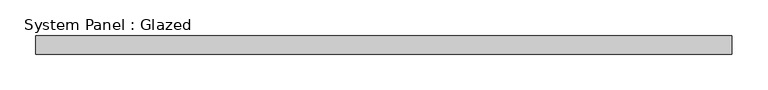
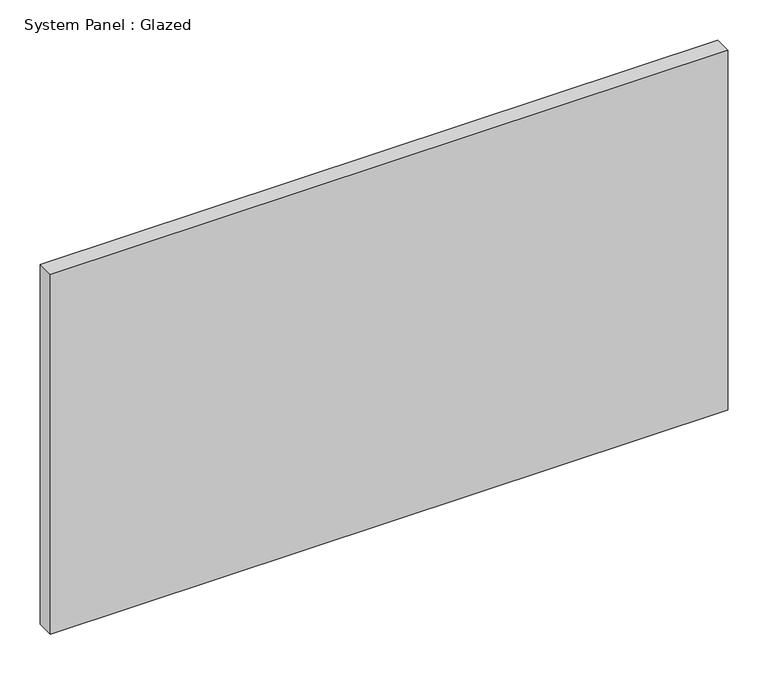
"""IFC4 building model written with IfcOpenShell, lengths in millimetres: plate geometry, System Panel : Glazed."""

from ifc_helpers import new_model, si_unit, origin, origin_with_axes, place, context, project, spatial, polyline, outline, extrude, source, transform, mapped, element, save


def system_panel_glazed_55a8196a(model_context):
    return source(origin(), model_context, "Body", "SweptSolid", [
        extrude(outline(polyline([(485.775, 19.05), (-485.775, 19.05), (-485.775, 44.45), (485.775, 44.45), (485.775, 19.05)])), origin_with_axes(), (0.0, 0.0, 1.0), 546.1),
    ])


if __name__ == "__main__":
    model = new_model("IFC4")
    model_context = context("Model", 3, world=origin())
    ifc_project = project(units=[si_unit("LENGTHUNIT", "METRE", prefix="MILLI")], contexts=[model_context])
    site = spatial("IfcSite", under=ifc_project)
    building = spatial("IfcBuilding", under=site)
    placement = place(None, origin())
    system_panel_glazed_shape = system_panel_glazed_55a8196a(model_context)
    element("IfcPlate", 1, ObjectType="System Panel : Glazed", at=placement, inside=building, context=model_context, shape_type="MappedRepresentation", body=[
        mapped(system_panel_glazed_shape, transform((0.0, 0.0, 0.0), x_axis=(1.0, 0.0, 0.0), y_axis=(0.0, 1.0, 0.0), z_axis=(0.0, 0.0, 1.0))),
    ])
    save(model, "model.ifc")

# Revit data of these elements
# Type "System Panel : Glazed"
#   Construction Type Id = "GSP4R"
#   Analytic Construction = "1/8 in Pilkington single glazing"
#   Visual Light Transmittance = 0.9
#   Solar Heat Gain Coefficient = 0.86
#   Heat Transfer Coefficient (U) = 1.18115 BTU/(h·ft²·°F)
# Element 1 (IfcPlate, "System Panel : Glazed")
#   Materials on its faces: "Glass"
# Materials
#   "Glass": class "Glass", colour RGB 0 128 192, transparency 0.75, Description = "Soda Lime Glass", Cost = 0
